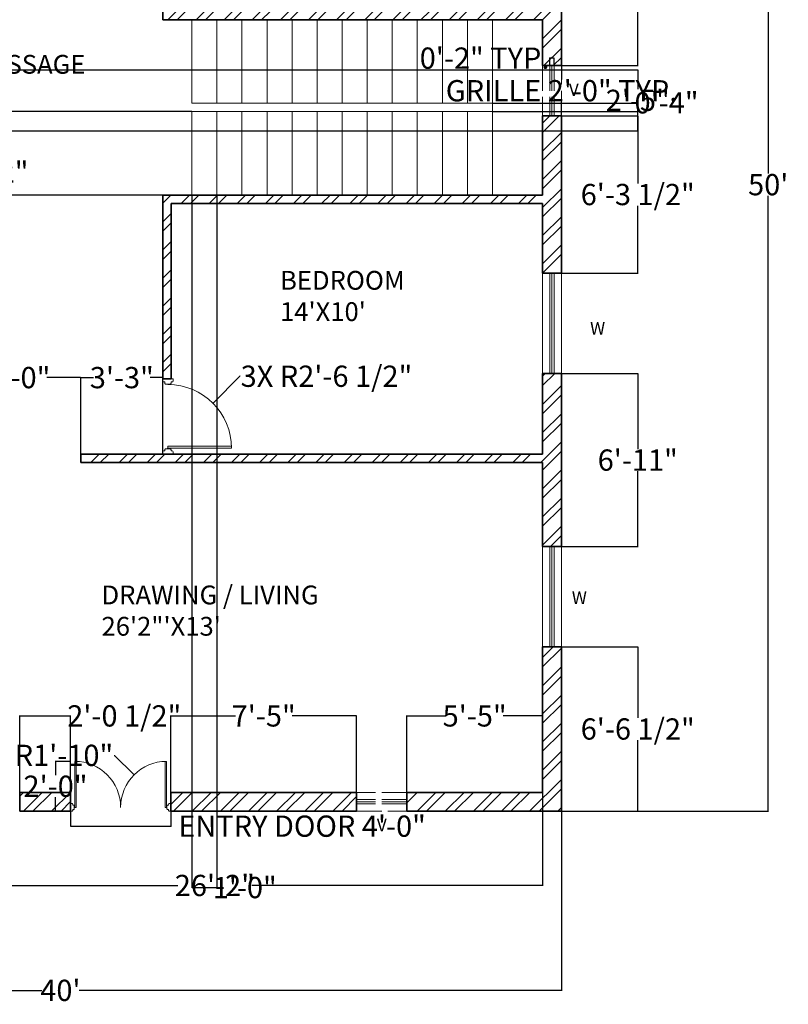
# Model space of a CAD drawing. Units: inches. Extents: x 1583 to 2239, y 1430 to 2174.
# Tile 4 of 5: x 1871 to 2239, y 1430 to 1902. Entities that reach past the tile are written whole.
import ezdxf

# ---------------------------------------------------------------- set-up
doc = ezdxf.new("R2010")
doc.units = ezdxf.units.IN
doc.linetypes.add('ACAD_ISO02W100', pattern=[15, 12, -3])
for name, color, linetype, lineweight in [('00 FURNITURE', 15, 'Continuous', 15), ('A-ANNO-DIMS', 2, 'Continuous', 18), ('A-ANNO-TEXT', 7, 'Continuous', 18), ('A-AREA-IDEN', 7, 'Continuous', 25), ('A-DOOR', 3, 'Continuous', 18), ('A-FLOR-STRS', 7, 'Continuous', 18), ('A-GLAZ-VENT', 6, 'ACAD_ISO02W100', 13), ('A-WALL-PATT', 252, 'Continuous', 13), ('WALL', 7, 'Continuous', 35), ('WINDOW', 160, 'Continuous', 18)]:
    doc.layers.add(name, color=color, linetype=linetype, lineweight=lineweight)
doc.styles.get("Standard").update_dxf_attribs({"font": 'arial.ttf'})
doc.dimstyles.get("Standard").update_dxf_attribs({"dimtxt": 10.18, "dimasz": 0.18, "dimexe": 0.18, "dimexo": 0.0625, "dimgap": 0.09, "dimtad": 0, "dimtih": 1, "dimtoh": 1, "dimdec": 0, "dimzin": 0, "dimdsep": 46, "dimlunit": 3, "dimtxsty": 'Standard', "dimcen": 0.09, "dimadec": 0, "dimazin": 0, "dimtfac": 1, "dimtdec": 0, "dimtofl": 0, "dimtmove": 0, "dimatfit": 3, "dimfxl": 1, "dimtolj": 1, "dimtzin": 0, "dimarcsym": 0})

# ---------------------------------------------------------------- blocks, each defined once
blk = doc.blocks.new('DDD')
at = {"layer": '00 FURNITURE'}
for p, q in [((-12579.77, -15859.53), (-12579.77, -15829.05)), ((-12578.77, -15859.53), (-12578.77, -15829.03)), ((-12612.02, -15857.03), (-12612.02, -15862.03)), ((-12611.02, -15857.03), (-12612.02, -15857.03)), ((-12610.52, -15858.03), (-12610.52, -15857.53)), ((-12610.52, -15861.53), (-12610.52, -15861.03)), ((-12578.77, -15859.53), (-12579.77, -15859.53)), ((-12577.52, -15858.03), (-12577.52, -15857.53)), ((-12577.52, -15861.53), (-12577.52, -15861.03)), ((-12577.02, -15857.03), (-12576.02, -15857.03)), ((-12576.02, -15857.03), (-12576.02, -15862.03)), ((-12612.02, -15862.03), (-12611.02, -15862.03)), ((-12576.02, -15862.03), (-12577.02, -15862.03))]:
    blk.add_line(p, q, dxfattribs=at)
for points in [[(-12610.52, -15861.03), (-12610.02, -15861.03, 0.414214), (-12609.52, -15860.53), (-12609.52, -15858.53, 0.414214), (-12610.02, -15858.03), (-12610.52, -15858.03)], [(-12577.52, -15861.03), (-12578.02, -15861.03, -0.414214), (-12578.52, -15860.53), (-12578.52, -15858.53, -0.414214), (-12578.02, -15858.03), (-12577.52, -15858.03)]]:
    blk.add_lwpolyline(points, format="xyb", dxfattribs=at)
for centre, radius, start, end in [((-12578.77, -15859.53), 30.5, 90, 180), ((-12611.02, -15857.53), 0.5, 0, 90), ((-12577.02, -15857.53), 0.5, 90, 180), ((-12611.02, -15861.53), 0.5, 270, 0), ((-12577.02, -15861.53), 0.5, 180, 270)]:
    blk.add_arc(centre, radius, start, end, dxfattribs=at)
blk = doc.blocks.new('*D3')
at = {"layer": 'A-ANNO-DIMS', "color": 0, "lineweight": -2, "transparency": 16777216}
for p, q in [((1807.53, 1531.58), (1807.53, 1486.86)), ((2121.53, 1531.58), (2121.53, 1486.86)), ((1807.71, 1487.04), (1946.87, 1487.04)), ((2121.35, 1487.04), (1982.19, 1487.04))]:
    blk.add_line(p, q, dxfattribs=at)
at = {"layer": 'A-ANNO-DIMS', "color": 0, "transparency": 16777216}
for points in [[(1807.71, 1487.07), (1807.71, 1487.01), (1807.53, 1487.04)], [(2121.35, 1487.07), (2121.35, 1487.01), (2121.53, 1487.04)]]:
    blk.add_solid(points, dxfattribs=at)
at = {"layer": 'Defpoints', "color": 0, "transparency": 16777216}
for p in [(1807.53, 1531.64), (2121.53, 1531.64), (2121.53, 1487.04)]:
    blk.add_point(p, dxfattribs=at)
at = {"layer": 'A-ANNO-DIMS', "color": 0, "transparency": 16777216, "insert": (1964.53, 1487.04), "char_height": 10.18, "attachment_point": 5}
blk.add_mtext('\\A1;26\'-2"', dxfattribs=at)
blk = doc.blocks.new('PUJA')
at = {"layer": '00 FURNITURE'}
for p, q in [((-1941.8, -16091.75), (-1938.89, -16091.75)), ((-1941.8, -16092.33), (-1941.8, -16091.75)), ((-1938.89, -16091.75), (-1938.89, -16092.33)), ((-1940.35, -16093.35), (-1958.14, -16093.35)), ((-1940.35, -16093.93), (-1958.13, -16093.93)), ((-1941.22, -16092.62), (-1941.51, -16092.62)), ((-1940.35, -16093.35), (-1940.35, -16093.93)), ((-1939.18, -16092.62), (-1939.47, -16092.62)), ((-1940.35, -16128.93), (-1958.14, -16128.93)), ((-1940.35, -16128.35), (-1958.13, -16128.35)), ((-1941.8, -16129.96), (-1941.8, -16130.54)), ((-1941.22, -16129.66), (-1941.51, -16129.66)), ((-1940.35, -16128.93), (-1940.35, -16128.35)), ((-1939.18, -16129.66), (-1939.47, -16129.66)), ((-1938.89, -16130.54), (-1938.89, -16129.96)), ((-1941.8, -16130.54), (-1938.89, -16130.54))]:
    blk.add_line(p, q, dxfattribs=at)
for points in [[(-1939.47, -16092.62), (-1939.47, -16092.91, -0.414214), (-1939.76, -16093.21), (-1940.93, -16093.21, -0.414214), (-1941.22, -16092.91), (-1941.22, -16092.62)], [(-1939.47, -16129.66), (-1939.47, -16129.37, 0.414214), (-1939.76, -16129.08), (-1940.93, -16129.08, 0.414214), (-1941.22, -16129.37), (-1941.22, -16129.66)]]:
    blk.add_lwpolyline(points, format="xyb", dxfattribs=at)
for centre, radius, start, end in [((-1940.35, -16093.35), 17.79, 180, 270), ((-1941.51, -16092.33), 0.292, 180, 270), ((-1939.18, -16092.33), 0.292, 270, 0), ((-1940.35, -16128.93), 17.79, 90, 180), ((-1941.51, -16129.96), 0.292, 90, 180), ((-1939.18, -16129.96), 0.292, 0, 90)]:
    blk.add_arc(centre, radius, start, end, dxfattribs=at)
blk = doc.blocks.new('*D9')
at = {"layer": 'A-ANNO-DIMS', "color": 0, "lineweight": -2, "transparency": 16777216}
for p, q in [((1650.53, 1522.58), (1650.53, 1436.63)), ((2130.53, 1522.58), (2130.53, 1436.63)), ((1650.71, 1436.81), (1881.6, 1436.81)), ((2130.35, 1436.81), (1899.47, 1436.81))]:
    blk.add_line(p, q, dxfattribs=at)
at = {"layer": 'A-ANNO-DIMS', "color": 0, "transparency": 16777216}
for points in [[(1650.71, 1436.84), (1650.71, 1436.78), (1650.53, 1436.81)], [(2130.35, 1436.84), (2130.35, 1436.78), (2130.53, 1436.81)]]:
    blk.add_solid(points, dxfattribs=at)
at = {"layer": 'Defpoints', "color": 0, "transparency": 16777216}
for p in [(1650.53, 1522.64), (2130.53, 1522.64), (2130.53, 1436.81)]:
    blk.add_point(p, dxfattribs=at)
at = {"layer": 'A-ANNO-DIMS', "color": 0, "transparency": 16777216, "insert": (1890.53, 1436.81), "char_height": 10.18, "attachment_point": 5}
blk.add_mtext("\\A1;40'", dxfattribs=at)
blk = doc.blocks.new('*D10')
at = {"layer": 'A-ANNO-DIMS', "color": 0, "lineweight": -2, "transparency": 16777216}
for p, q in [((2130.59, 2122.64), (2229.81, 2122.64)), ((2229.63, 2122.46), (2229.63, 1827.93)), ((2229.63, 1522.82), (2229.63, 1817.35)), ((2130.59, 1522.64), (2229.81, 1522.64))]:
    blk.add_line(p, q, dxfattribs=at)
at = {"layer": 'A-ANNO-DIMS', "color": 0, "transparency": 16777216}
for points in [[(2229.6, 2122.46), (2229.66, 2122.46), (2229.63, 2122.64)], [(2229.6, 1522.82), (2229.66, 1522.82), (2229.63, 1522.64)]]:
    blk.add_solid(points, dxfattribs=at)
at = {"layer": 'Defpoints', "color": 0, "transparency": 16777216}
for p in [(2130.53, 2122.64), (2130.53, 1522.64), (2229.63, 1522.64)]:
    blk.add_point(p, dxfattribs=at)
at = {"layer": 'A-ANNO-DIMS', "color": 0, "transparency": 16777216, "insert": (2229.63, 1822.64), "char_height": 10.18, "attachment_point": 5}
blk.add_mtext("\\A1;50'", dxfattribs=at)
blk = doc.blocks.new('WIN-SASH-48IN')
for p, q in [((48, 2), (0, 2)), ((48, 1), (0, 1)), ((48, 0), (0, 0))]:
    blk.add_line(p, q)
blk = doc.blocks.new('VENT-GRILLE-24IN')
for p, q in [((24, 2), (0, 2)), ((24, 1), (0, 1)), ((24, 0), (0, 0))]:
    blk.add_line(p, q)
blk = doc.blocks.new('*D15')
at = {"layer": 'A-ANNO-DIMS', "color": 0, "lineweight": -2, "transparency": 16777216}
for p, q in [((2127.09, 1879.63), (2130.81, 1879.63)), ((2130.63, 1879.45), (2130.63, 1872.98)), ((2130.63, 1855.81), (2130.63, 1862.27)), ((2127.09, 1855.63), (2130.81, 1855.63))]:
    blk.add_line(p, q, dxfattribs=at)
at = {"layer": 'A-ANNO-DIMS', "color": 0, "transparency": 16777216}
for points in [[(2130.6, 1879.45), (2130.66, 1879.45), (2130.63, 1879.63)], [(2130.6, 1855.81), (2130.66, 1855.81), (2130.63, 1855.63)]]:
    blk.add_solid(points, dxfattribs=at)
at = {"layer": 'Defpoints', "color": 0, "transparency": 16777216}
for p in [(2127.03, 1879.63), (2130.63, 1879.63), (2127.03, 1855.63)]:
    blk.add_point(p, dxfattribs=at)
at = {"layer": 'A-ANNO-DIMS', "color": 0, "transparency": 16777216, "insert": (2130.63, 1867.63), "char_height": 10.18, "attachment_point": 5}
blk.add_mtext('\\A1;GRILLE 2\'-0" TYP.', dxfattribs=at)
blk = doc.blocks.new('*D16')
at = {"layer": 'A-ANNO-DIMS', "color": 0, "lineweight": -2, "transparency": 16777216}
for p, q in [((2125.03, 1883.23), (2124.85, 1883.23)), ((2125.03, 1879.69), (2125.03, 1883.41)), ((2126.85, 1883.23), (2125.21, 1883.23)), ((2127.03, 1879.69), (2127.03, 1883.41))]:
    blk.add_line(p, q, dxfattribs=at)
at = {"layer": 'A-ANNO-DIMS', "color": 0, "transparency": 16777216}
for points in [[(2125.21, 1883.26), (2125.21, 1883.2), (2125.03, 1883.23)], [(2126.85, 1883.26), (2126.85, 1883.2), (2127.03, 1883.23)]]:
    blk.add_solid(points, dxfattribs=at)
at = {"layer": 'Defpoints', "color": 0, "transparency": 16777216}
for p in [(2125.03, 1883.23), (2125.03, 1879.63), (2127.03, 1879.63)]:
    blk.add_point(p, dxfattribs=at)
at = {"layer": 'A-ANNO-DIMS', "color": 0, "transparency": 16777216, "insert": (2093.74, 1883.23), "char_height": 10.18, "attachment_point": 5}
blk.add_mtext('\\A1;0\'-2" TYP.', dxfattribs=at)
blk = doc.blocks.new('*D27')
at = {"layer": 'A-ANNO-DIMS', "color": 0, "lineweight": -2, "transparency": 16777216}
for p, q in [((1895.39, 1522.58), (1895.39, 1515.26)), ((1943.39, 1522.58), (1943.39, 1515.26)), ((1895.57, 1515.44), (1943.21, 1515.44)), ((1943.39, 1515.44), (1943.57, 1515.44))]:
    blk.add_line(p, q, dxfattribs=at)
at = {"layer": 'A-ANNO-DIMS', "color": 0, "transparency": 16777216}
for points in [[(1895.57, 1515.47), (1895.57, 1515.41), (1895.39, 1515.44)], [(1943.21, 1515.47), (1943.21, 1515.41), (1943.39, 1515.44)]]:
    blk.add_solid(points, dxfattribs=at)
at = {"layer": 'Defpoints', "color": 0, "transparency": 16777216}
for p in [(1895.39, 1522.64), (1943.39, 1522.64), (1943.39, 1515.44)]:
    blk.add_point(p, dxfattribs=at)
at = {"layer": 'A-ANNO-DIMS', "color": 0, "transparency": 16777216, "insert": (2006.31, 1515.44), "char_height": 10.18, "attachment_point": 5}
blk.add_mtext('\\A1;ENTRY DOOR 4\'-0"', dxfattribs=at)
blk = doc.blocks.new('*D28')
at = {"layer": 'A-ANNO-DIMS', "color": 0, "lineweight": -2, "transparency": 16777216}
for p, q in [((1895.33, 1546.46), (1888.01, 1546.46)), ((1888.19, 1546.28), (1888.19, 1539.84)), ((1888.19, 1522.82), (1888.19, 1529.26)), ((1895.33, 1522.64), (1888.01, 1522.64))]:
    blk.add_line(p, q, dxfattribs=at)
at = {"layer": 'A-ANNO-DIMS', "color": 0, "transparency": 16777216}
for points in [[(1888.16, 1546.28), (1888.22, 1546.28), (1888.19, 1546.46)], [(1888.16, 1522.82), (1888.22, 1522.82), (1888.19, 1522.64)]]:
    blk.add_solid(points, dxfattribs=at)
at = {"layer": 'Defpoints', "color": 0, "transparency": 16777216}
for p in [(1895.39, 1546.46), (1888.19, 1522.64), (1895.39, 1522.64)]:
    blk.add_point(p, dxfattribs=at)
at = {"layer": 'A-ANNO-DIMS', "color": 0, "transparency": 16777216, "insert": (1888.19, 1534.55), "char_height": 10.18, "attachment_point": 5}
blk.add_mtext('\\A1;2\'-0"', dxfattribs=at)
blk = doc.blocks.new('*D33')
at = {"layer": 'A-ANNO-DIMS', "color": 0, "lineweight": -2, "transparency": 16777216}
for p, q in [((2056.46, 1531.7), (2056.46, 1568.42)), ((2056.64, 1568.24), (2075.38, 1568.24)), ((2121.35, 1568.24), (2102.62, 1568.24)), ((2121.53, 1531.7), (2121.53, 1568.42))]:
    blk.add_line(p, q, dxfattribs=at)
at = {"layer": 'A-ANNO-DIMS', "color": 0, "transparency": 16777216}
for points in [[(2056.64, 1568.27), (2056.64, 1568.21), (2056.46, 1568.24)], [(2121.35, 1568.27), (2121.35, 1568.21), (2121.53, 1568.24)]]:
    blk.add_solid(points, dxfattribs=at)
at = {"layer": 'Defpoints', "color": 0, "transparency": 16777216}
for p in [(2121.53, 1568.24), (2056.46, 1531.64), (2121.53, 1531.64)]:
    blk.add_point(p, dxfattribs=at)
at = {"layer": 'A-ANNO-DIMS', "color": 0, "transparency": 16777216, "insert": (2089, 1568.24), "char_height": 10.18, "attachment_point": 5}
blk.add_mtext('\\A1;5\'-5"', dxfattribs=at)
blk = doc.blocks.new('*D34')
at = {"layer": 'A-ANNO-DIMS', "color": 0, "lineweight": -2, "transparency": 16777216}
for p, q in [((1871.02, 1531.7), (1871.02, 1568.42)), ((1871.2, 1568.24), (1895.21, 1568.24)), ((1895.39, 1531.7), (1895.39, 1568.42)), ((1895.39, 1568.24), (1895.57, 1568.24))]:
    blk.add_line(p, q, dxfattribs=at)
at = {"layer": 'A-ANNO-DIMS', "color": 0, "transparency": 16777216}
for points in [[(1871.2, 1568.27), (1871.2, 1568.21), (1871.02, 1568.24)], [(1895.21, 1568.27), (1895.21, 1568.21), (1895.39, 1568.24)]]:
    blk.add_solid(points, dxfattribs=at)
at = {"layer": 'Defpoints', "color": 0, "transparency": 16777216}
for p in [(1895.39, 1568.24), (1871.02, 1531.64), (1895.39, 1531.64)]:
    blk.add_point(p, dxfattribs=at)
at = {"layer": 'A-ANNO-DIMS', "color": 0, "transparency": 16777216, "insert": (1921.14, 1568.24), "char_height": 10.18, "attachment_point": 5}
blk.add_mtext('\\A1;2\'-0 1/2"', dxfattribs=at)
blk = doc.blocks.new('*D35')
at = {"layer": 'A-ANNO-DIMS', "color": 0, "lineweight": -2, "transparency": 16777216}
for p, q in [((1943.39, 1531.7), (1943.39, 1568.42)), ((1943.57, 1568.24), (1974.35, 1568.24)), ((2032.28, 1568.24), (2001.51, 1568.24)), ((2032.46, 1531.7), (2032.46, 1568.42))]:
    blk.add_line(p, q, dxfattribs=at)
at = {"layer": 'A-ANNO-DIMS', "color": 0, "transparency": 16777216}
for points in [[(1943.57, 1568.27), (1943.57, 1568.21), (1943.39, 1568.24)], [(2032.28, 1568.27), (2032.28, 1568.21), (2032.46, 1568.24)]]:
    blk.add_solid(points, dxfattribs=at)
at = {"layer": 'Defpoints', "color": 0, "transparency": 16777216}
for p in [(2032.46, 1568.24), (1943.39, 1531.64), (2032.46, 1531.64)]:
    blk.add_point(p, dxfattribs=at)
at = {"layer": 'A-ANNO-DIMS', "color": 0, "transparency": 16777216, "insert": (1987.93, 1568.24), "char_height": 10.18, "attachment_point": 5}
blk.add_mtext('\\A1;7\'-5"', dxfattribs=at)
blk = doc.blocks.new('*D40')
at = {"layer": 'A-ANNO-DIMS', "color": 0, "lineweight": -2, "transparency": 16777216}
for p, q in [((2130.59, 1601.31), (2167.31, 1601.31)), ((2167.13, 1601.13), (2167.13, 1567.33)), ((2167.13, 1522.82), (2167.13, 1556.62)), ((2130.59, 1522.64), (2167.31, 1522.64))]:
    blk.add_line(p, q, dxfattribs=at)
at = {"layer": 'A-ANNO-DIMS', "color": 0, "transparency": 16777216}
for points in [[(2167.1, 1601.13), (2167.16, 1601.13), (2167.13, 1601.31)], [(2167.1, 1522.82), (2167.16, 1522.82), (2167.13, 1522.64)]]:
    blk.add_solid(points, dxfattribs=at)
at = {"layer": 'Defpoints', "color": 0, "transparency": 16777216}
for p in [(2130.53, 1601.31), (2167.13, 1601.31), (2130.53, 1522.64)]:
    blk.add_point(p, dxfattribs=at)
at = {"layer": 'A-ANNO-DIMS', "color": 0, "transparency": 16777216, "insert": (2167.13, 1561.97), "char_height": 10.18, "attachment_point": 5}
blk.add_mtext('\\A1;6\'-6 1/2"', dxfattribs=at)
blk = doc.blocks.new('*D41')
at = {"layer": 'A-ANNO-DIMS', "color": 0, "lineweight": -2, "transparency": 16777216}
for p, q in [((2130.59, 1732.2), (2167.31, 1732.2)), ((2167.13, 1732.02), (2167.13, 1696.04)), ((2167.13, 1649.49), (2167.13, 1685.47)), ((2130.59, 1649.31), (2167.31, 1649.31))]:
    blk.add_line(p, q, dxfattribs=at)
at = {"layer": 'A-ANNO-DIMS', "color": 0, "transparency": 16777216}
for points in [[(2167.1, 1732.02), (2167.16, 1732.02), (2167.13, 1732.2)], [(2167.1, 1649.49), (2167.16, 1649.49), (2167.13, 1649.31)]]:
    blk.add_solid(points, dxfattribs=at)
at = {"layer": 'Defpoints', "color": 0, "transparency": 16777216}
for p in [(2130.53, 1732.2), (2167.13, 1732.2), (2130.53, 1649.31)]:
    blk.add_point(p, dxfattribs=at)
at = {"layer": 'A-ANNO-DIMS', "color": 0, "transparency": 16777216, "insert": (2167.13, 1690.75), "char_height": 10.18, "attachment_point": 5}
blk.add_mtext('\\A1;6\'-11"', dxfattribs=at)
blk = doc.blocks.new('*D42')
at = {"layer": 'A-ANNO-DIMS', "color": 0, "lineweight": -2, "transparency": 16777216}
for p, q in [((2130.59, 1855.63), (2167.31, 1855.63)), ((2167.13, 1855.45), (2167.13, 1823.27)), ((2167.13, 1780.38), (2167.13, 1812.55)), ((2130.59, 1780.2), (2167.31, 1780.2))]:
    blk.add_line(p, q, dxfattribs=at)
at = {"layer": 'A-ANNO-DIMS', "color": 0, "transparency": 16777216}
for points in [[(2167.1, 1855.45), (2167.16, 1855.45), (2167.13, 1855.63)], [(2167.1, 1780.38), (2167.16, 1780.38), (2167.13, 1780.2)]]:
    blk.add_solid(points, dxfattribs=at)
at = {"layer": 'Defpoints', "color": 0, "transparency": 16777216}
for p in [(2130.53, 1855.63), (2167.13, 1855.63), (2130.53, 1780.2)]:
    blk.add_point(p, dxfattribs=at)
at = {"layer": 'A-ANNO-DIMS', "color": 0, "transparency": 16777216, "insert": (2167.13, 1817.91), "char_height": 10.18, "attachment_point": 5}
blk.add_mtext('\\A1;6\'-3 1/2"', dxfattribs=at)
blk = doc.blocks.new('*D43')
at = {"layer": 'A-ANNO-DIMS', "color": 0, "lineweight": -2, "transparency": 16777216}
for p, q in [((2130.59, 1965.82), (2167.31, 1965.82)), ((2167.13, 1965.64), (2167.13, 1927.92)), ((2167.13, 1879.81), (2167.13, 1917.52)), ((2130.59, 1879.63), (2167.31, 1879.63))]:
    blk.add_line(p, q, dxfattribs=at)
at = {"layer": 'A-ANNO-DIMS', "color": 0, "transparency": 16777216}
for points in [[(2167.1, 1965.64), (2167.16, 1965.64), (2167.13, 1965.82)], [(2167.1, 1879.81), (2167.16, 1879.81), (2167.13, 1879.63)]]:
    blk.add_solid(points, dxfattribs=at)
at = {"layer": 'Defpoints', "color": 0, "transparency": 16777216}
for p in [(2130.53, 1965.82), (2167.13, 1965.82), (2130.53, 1879.63)]:
    blk.add_point(p, dxfattribs=at)
at = {"layer": 'A-ANNO-DIMS', "color": 0, "transparency": 16777216, "insert": (2167.13, 1922.72), "char_height": 10.18, "attachment_point": 5}
blk.add_mtext('\\A1;7\'-2"', dxfattribs=at)
blk = doc.blocks.new('*D44')
at = {"layer": 'A-ANNO-DIMS', "color": 0, "lineweight": -2, "transparency": 16777216}
for p, q in [((1953.47, 1857.64), (1613.75, 1857.64)), ((1613.93, 1857.46), (1613.93, 1842.93)), ((1613.93, 1817.82), (1613.93, 1832.35)), ((1953.47, 1817.64), (1613.75, 1817.64))]:
    blk.add_line(p, q, dxfattribs=at)
at = {"layer": 'A-ANNO-DIMS', "color": 0, "transparency": 16777216}
for points in [[(1613.9, 1857.46), (1613.96, 1857.46), (1613.93, 1857.64)], [(1613.9, 1817.82), (1613.96, 1817.82), (1613.93, 1817.64)]]:
    blk.add_solid(points, dxfattribs=at)
at = {"layer": 'Defpoints', "color": 0, "transparency": 16777216}
for p in [(1613.93, 1857.64), (1953.53, 1857.64), (1953.53, 1817.64)]:
    blk.add_point(p, dxfattribs=at)
at = {"layer": 'A-ANNO-DIMS', "color": 0, "transparency": 16777216, "insert": (1613.93, 1837.64), "char_height": 10.18, "attachment_point": 5}
blk.add_mtext('\\A1;3\'-4"', dxfattribs=at)
blk = doc.blocks.new('*D45')
at = {"layer": 'A-ANNO-DIMS', "color": 0, "lineweight": -2, "transparency": 16777216}
for p, q in [((2097.59, 1861.64), (2167.31, 1861.64)), ((2167.13, 1861.64), (2167.13, 1861.82)), ((2167.13, 1861.82), (2167.31, 1861.82)), ((2167.13, 1857.82), (2167.13, 1861.46)), ((2097.59, 1857.64), (2167.31, 1857.64))]:
    blk.add_line(p, q, dxfattribs=at)
at = {"layer": 'A-ANNO-DIMS', "color": 0, "transparency": 16777216}
for points in [[(2167.1, 1861.46), (2167.16, 1861.46), (2167.13, 1861.64)], [(2167.1, 1857.82), (2167.16, 1857.82), (2167.13, 1857.64)]]:
    blk.add_solid(points, dxfattribs=at)
at = {"layer": 'Defpoints', "color": 0, "transparency": 16777216}
for p in [(2097.53, 1861.64), (2167.13, 1861.64), (2097.53, 1857.64)]:
    blk.add_point(p, dxfattribs=at)
at = {"layer": 'A-ANNO-DIMS', "color": 0, "transparency": 16777216, "insert": (2180.93, 1861.82), "char_height": 10.18, "attachment_point": 5}
blk.add_mtext('\\A1;0\'-4"', dxfattribs=at)
blk = doc.blocks.new('*D47')
at = {"layer": 'A-ANNO-DIMS', "color": 0, "lineweight": -2, "transparency": 16777216}
for p, q in [((1953.53, 1817.58), (1953.53, 1485.86)), ((1965.53, 1817.58), (1965.53, 1485.86)), ((1953.71, 1486.04), (1965.35, 1486.04)), ((1965.53, 1486.04), (1965.71, 1486.04))]:
    blk.add_line(p, q, dxfattribs=at)
at = {"layer": 'A-ANNO-DIMS', "color": 0, "transparency": 16777216}
for points in [[(1953.71, 1486.07), (1953.71, 1486.01), (1953.53, 1486.04)], [(1965.35, 1486.07), (1965.35, 1486.01), (1965.53, 1486.04)]]:
    blk.add_solid(points, dxfattribs=at)
at = {"layer": 'Defpoints', "color": 0, "transparency": 16777216}
for p in [(1953.53, 1817.64), (1965.53, 1817.64), (1965.53, 1486.04)]:
    blk.add_point(p, dxfattribs=at)
at = {"layer": 'A-ANNO-DIMS', "color": 0, "transparency": 16777216, "insert": (1978.85, 1486.04), "char_height": 10.18, "attachment_point": 5}
blk.add_mtext('\\A1;1\'-0"', dxfattribs=at)
blk = doc.blocks.new('*D51')
at = {"layer": 'A-ANNO-DIMS', "color": 0, "lineweight": -2, "transparency": 16777216}
for p, q in [((1840.39, 1693.7), (1840.39, 1730.42)), ((1840.57, 1730.24), (1856.77, 1730.24)), ((1900.21, 1730.24), (1884.01, 1730.24)), ((1900.39, 1693.7), (1900.39, 1730.42))]:
    blk.add_line(p, q, dxfattribs=at)
at = {"layer": 'A-ANNO-DIMS', "color": 0, "transparency": 16777216}
for points in [[(1840.57, 1730.27), (1840.57, 1730.21), (1840.39, 1730.24)], [(1900.21, 1730.27), (1900.21, 1730.21), (1900.39, 1730.24)]]:
    blk.add_solid(points, dxfattribs=at)
at = {"layer": 'Defpoints', "color": 0, "transparency": 16777216}
for p in [(1900.39, 1730.24), (1840.39, 1693.64), (1900.39, 1693.64)]:
    blk.add_point(p, dxfattribs=at)
at = {"layer": 'A-ANNO-DIMS', "color": 0, "transparency": 16777216, "insert": (1870.39, 1730.24), "char_height": 10.18, "attachment_point": 5}
blk.add_mtext('\\A1;5\'-0"', dxfattribs=at)
blk = doc.blocks.new('*D56')
at = {"layer": 'A-ANNO-DIMS', "color": 0, "lineweight": -2, "transparency": 16777216}
for p, q in [((1803.59, 1877.64), (2167.31, 1877.64)), ((2167.13, 1877.46), (2167.13, 1868.3)), ((2167.13, 1848.57), (2167.13, 1857.73)), ((1802.65, 1848.39), (2167.31, 1848.39))]:
    blk.add_line(p, q, dxfattribs=at)
at = {"layer": 'A-ANNO-DIMS', "color": 0, "transparency": 16777216}
for points in [[(2167.1, 1877.46), (2167.16, 1877.46), (2167.13, 1877.64)], [(2167.1, 1848.57), (2167.16, 1848.57), (2167.13, 1848.39)]]:
    blk.add_solid(points, dxfattribs=at)
at = {"layer": 'Defpoints', "color": 0, "transparency": 16777216}
for p in [(1803.53, 1877.64), (1802.59, 1848.39), (2167.13, 1848.39)]:
    blk.add_point(p, dxfattribs=at)
at = {"layer": 'A-ANNO-DIMS', "color": 0, "transparency": 16777216, "insert": (2167.13, 1863.01), "char_height": 10.18, "attachment_point": 5}
blk.add_mtext('\\A1;2\'-5"', dxfattribs=at)
blk = doc.blocks.new('*D57')
at = {"layer": 'A-ANNO-DIMS', "color": 0, "lineweight": -2, "transparency": 16777216}
for p, q in [((1900.39, 1693.7), (1900.39, 1730.42)), ((1900.57, 1730.24), (1906.34, 1730.24)), ((1939.35, 1730.24), (1933.58, 1730.24)), ((1939.53, 1693.7), (1939.53, 1730.42))]:
    blk.add_line(p, q, dxfattribs=at)
at = {"layer": 'A-ANNO-DIMS', "color": 0, "transparency": 16777216}
for points in [[(1900.57, 1730.27), (1900.57, 1730.21), (1900.39, 1730.24)], [(1939.35, 1730.27), (1939.35, 1730.21), (1939.53, 1730.24)]]:
    blk.add_solid(points, dxfattribs=at)
at = {"layer": 'Defpoints', "color": 0, "transparency": 16777216}
for p in [(1939.53, 1730.24), (1900.39, 1693.64), (1939.53, 1693.64)]:
    blk.add_point(p, dxfattribs=at)
at = {"layer": 'A-ANNO-DIMS', "color": 0, "transparency": 16777216, "insert": (1919.96, 1730.24), "char_height": 10.18, "attachment_point": 5}
blk.add_mtext('\\A1;3\'-3"', dxfattribs=at)
blk = doc.blocks.new('*D61')
at = {"layer": 'A-ANNO-DIMS', "color": 0, "lineweight": -2, "transparency": 16777216}
for p, q in [((1976.54, 1730.9), (1963.73, 1718.08)), ((1976.72, 1730.9), (1976.54, 1730.9)), ((1941.94, 1696.39), (1942.12, 1696.39)), ((1942.03, 1696.3), (1942.03, 1696.48))]:
    blk.add_line(p, q, dxfattribs=at)
at = {"layer": 'A-ANNO-DIMS', "color": 0, "transparency": 16777216}
blk.add_solid([(1963.7, 1718.1), (1963.75, 1718.06), (1963.6, 1717.96)], dxfattribs=at)
at = {"layer": 'Defpoints', "color": 0, "transparency": 16777216}
for p in [(1963.6, 1717.96), (1942.03, 1696.39)]:
    blk.add_point(p, dxfattribs=at)
at = {"layer": 'A-ANNO-DIMS', "color": 0, "transparency": 16777216, "insert": (2018, 1730.9), "char_height": 10.18, "attachment_point": 5}
blk.add_mtext('\\A1;3X R2\'-6 1/2"', dxfattribs=at)
blk = doc.blocks.new('*D63')
at = {"layer": 'A-ANNO-DIMS', "color": 0, "lineweight": -2, "transparency": 16777216}
for p, q in [((1916.32, 1549.35), (1916.5, 1549.35)), ((1916.5, 1549.35), (1925.71, 1540.14)), ((1941.32, 1524.44), (1941.5, 1524.44)), ((1941.41, 1524.35), (1941.41, 1524.53))]:
    blk.add_line(p, q, dxfattribs=at)
at = {"layer": 'A-ANNO-DIMS', "color": 0, "transparency": 16777216}
blk.add_solid([(1925.73, 1540.16), (1925.69, 1540.12), (1925.84, 1540.01)], dxfattribs=at)
at = {"layer": 'Defpoints', "color": 0, "transparency": 16777216}
for p in [(1925.84, 1540.01), (1941.41, 1524.44)]:
    blk.add_point(p, dxfattribs=at)
at = {"layer": 'A-ANNO-DIMS', "color": 0, "transparency": 16777216, "insert": (1882.85, 1549.35), "char_height": 10.18, "attachment_point": 5}
blk.add_mtext('\\A1;2X R1\'-10"', dxfattribs=at)
blk = doc.blocks.new('*D65')
at = {"layer": 'A-ANNO-DIMS', "color": 0, "lineweight": -2, "transparency": 16777216}
for p, q in [((1784.89, 1841.88), (1785.07, 1841.88)), ((1784.98, 1841.79), (1784.98, 1841.97)), ((1792.63, 1828.66), (1789.85, 1833.46)), ((1792.81, 1828.66), (1792.63, 1828.66))]:
    blk.add_line(p, q, dxfattribs=at)
at = {"layer": 'A-ANNO-DIMS', "color": 0, "transparency": 16777216}
blk.add_solid([(1789.88, 1833.48), (1789.83, 1833.45), (1789.76, 1833.62)], dxfattribs=at)
at = {"layer": 'Defpoints', "color": 0, "transparency": 16777216}
for p in [(1784.98, 1841.88), (1789.76, 1833.62)]:
    blk.add_point(p, dxfattribs=at)
at = {"layer": 'A-ANNO-DIMS', "color": 0, "transparency": 16777216, "insert": (1834.11, 1828.66), "char_height": 10.18, "attachment_point": 5}
blk.add_mtext('\\A1;8X R0\'-9 1/2"', dxfattribs=at)

msp = doc.modelspace()

# ---------------------------------------------------------------- hatches: boundary and pattern name
at = {"layer": 'A-WALL-PATT'}
h = msp.add_hatch(dxfattribs=at)
h.set_pattern_fill('ANSI32', color=256)
h.paths.add_polyline_path([(1715.9, 2122.64), (1650.53, 2122.64), (1650.53, 1975.26), (1659.53, 1975.26), (1659.53, 1975.26), (1659.53, 2013.64), (1803.53, 2013.64), (1803.53, 1917.64), (1807.53, 1917.64), (1807.53, 2013.64), (1839.53, 2013.64), (1839.53, 2017.64), (1659.53, 2017.64), (1659.53, 2113.64), (1715.9, 2113.64)])
h.paths.add_polyline_path([(1893.86, 2122.64), (1763.9, 2122.64), (1763.9, 2113.64), (1875.53, 2113.64), (1875.53, 2013.64), (1879.53, 2013.64), (1879.53, 2037.64), (1909.53, 2037.64), (1909.53, 2041.64), (1879.53, 2041.64), (1879.53, 2113.64), (1893.86, 2113.64)])
h.paths.add_polyline_path([(1999.8, 2122.64), (1917.86, 2122.64), (1917.86, 2113.64), (1939.53, 2113.64), (1939.53, 2037.64), (1939.53, 1941.64), (1943.53, 1941.64), (1943.53, 2049.64), (2091.53, 2049.64), (2091.53, 2053.64), (1943.53, 2053.64), (1943.53, 2113.64), (1999.8, 2113.64)])
h.paths.add_polyline_path([(2130.53, 2122.64), (2023.8, 2122.64), (2023.8, 2113.64), (2121.53, 2113.64), (2121.53, 2049.64), (2121.53, 2013.82), (2130.53, 2013.82), (2130.53, 2013.82)])
h.paths.add_polyline_path([(2130.53, 1965.82), (2121.53, 1965.82), (2121.53, 1905.64), (1944.53, 1905.64), (1944.53, 1905.64), (1939.53, 1905.64), (1939.53, 1901.64), (2121.53, 1901.64), (2121.53, 1879.63), (2130.53, 1879.63)])
h.paths.add_polyline_path([(2130.53, 1855.63), (2121.53, 1855.63), (2121.53, 1817.64), (1939.53, 1817.64), (1939.53, 1729.64), (1943.53, 1729.64), (1943.53, 1813.64), (2121.53, 1813.64), (2121.53, 1780.2), (2130.53, 1780.2), (2130.53, 1780.2)])
h.paths.add_polyline_path([(2130.53, 1732.2), (2121.53, 1732.2), (2121.53, 1693.64), (1944.53, 1693.64), (1944.53, 1693.64), (1939.53, 1693.64), (1900.39, 1693.64), (1900.39, 1689.64), (2121.53, 1689.64), (2121.53, 1649.31), (2130.53, 1649.31), (2130.53, 1649.31)])
h.paths.add_polyline_path([(2130.53, 1601.31), (2121.53, 1601.31), (2121.53, 1531.64), (2056.46, 1531.64), (2056.46, 1522.64), (2130.53, 1522.64)])
h.paths.add_polyline_path([(2032.46, 1531.64), (1943.39, 1531.64), (1943.39, 1526.25), (1943.39, 1526.25), (1943.39, 1522.64), (2032.46, 1522.64)])
h.paths.add_polyline_path([(1895.39, 1531.64), (1871.02, 1531.64), (1871.02, 1522.64), (1895.39, 1522.64)])
h.paths.add_polyline_path([(1847.02, 1531.64), (1807.53, 1531.64), (1807.53, 1653.64), (1803.53, 1653.64), (1803.53, 1531.64), (1750.06, 1531.64), (1750.06, 1522.64), (1847.02, 1522.64)])
h.paths.add_polyline_path([(1702.06, 1531.64), (1659.53, 1531.64), (1659.53, 1587.56), (1650.53, 1587.56), (1650.53, 1522.64), (1702.06, 1522.64)])
h.paths.add_polyline_path([(1659.53, 1927.26), (1650.53, 1927.26), (1650.53, 1843.95), (1659.53, 1843.95), (1659.53, 1877.64)])
h.paths.add_polyline_path([(1659.53, 1801.64), (1807.53, 1801.64), (1807.53, 1881.64), (1689.53, 1881.64), (1689.53, 1877.64), (1803.53, 1877.64), (1803.53, 1805.64), (1659.53, 1805.64), (1659.53, 1819.95), (1650.53, 1819.95), (1650.53, 1766.08), (1659.53, 1766.08)])
h.paths.add_polyline_path([(1659.53, 1742.08), (1650.53, 1742.08), (1650.53, 1635.56), (1659.53, 1635.56), (1659.53, 1635.56), (1659.53, 1689.64), (1807.53, 1689.64), (1840.39, 1689.64), (1840.39, 1693.64), (1807.53, 1693.64), (1807.53, 1771.64), (1803.53, 1771.64), (1803.53, 1693.64), (1786.54, 1693.64), (1786.54, 1693.64), (1768.55, 1693.64), (1659.53, 1693.64), (1659.53, 1701.64)])

# ---------------------------------------------------------------- linework, layer by layer
at = {"layer": 'A-FLOR-STRS'}
for p, q in [((1953.53, 1901.64), (1953.53, 1861.64)), ((1965.53, 1901.64), (1965.53, 1861.64)), ((1977.53, 1901.64), (1977.53, 1861.64)), ((1989.53, 1901.64), (1989.53, 1861.64)), ((2001.53, 1901.64), (2001.53, 1861.64)), ((2013.53, 1901.64), (2013.53, 1861.64)), ((2025.53, 1901.64), (2025.53, 1861.64)), ((2037.53, 1901.64), (2037.53, 1861.64)), ((2049.53, 1901.64), (2049.53, 1861.64)), ((2061.53, 1901.64), (2061.53, 1861.64)), ((2073.53, 1901.64), (2073.53, 1861.64)), ((2085.53, 1901.64), (2085.53, 1861.64)), ((2097.53, 1901.64), (2097.53, 1817.64)), ((2097.53, 1861.64), (1953.53, 1861.64)), ((2097.53, 1857.64), (1953.53, 1857.64)), ((1953.53, 1857.64), (1953.53, 1817.64)), ((1965.53, 1857.64), (1965.53, 1817.64)), ((1977.53, 1857.64), (1977.53, 1817.64)), ((1989.53, 1857.64), (1989.53, 1817.64)), ((2001.53, 1857.64), (2001.53, 1817.64)), ((2013.53, 1857.64), (2013.53, 1817.64)), ((2025.53, 1857.64), (2025.53, 1817.64)), ((2037.53, 1857.64), (2037.53, 1817.64)), ((2049.53, 1857.64), (2049.53, 1817.64)), ((2061.53, 1857.64), (2061.53, 1817.64)), ((2073.53, 1857.64), (2073.53, 1817.64)), ((2085.53, 1857.64), (2085.53, 1817.64))]:
    msp.add_line(p, q, dxfattribs=at)
at = {"layer": 'A-GLAZ-VENT'}
for points in [[(2121.53, 1855.63), (2130.53, 1855.63), (2130.53, 1879.63), (2121.53, 1879.63)], [(2032.46, 1531.64), (2032.46, 1522.64), (2056.46, 1522.64), (2056.46, 1531.64)]]:
    msp.add_lwpolyline(points, close=True, dxfattribs=at)
at = {"layer": 'WALL'}
for p, q in [((2130.53, 1965.82), (2130.53, 1879.63)), ((1939.53, 1901.64), (1939.53, 1905.64)), ((1939.53, 1901.64), (2121.53, 1901.64)), ((2121.53, 1901.64), (2121.53, 1879.63)), ((2121.53, 1879.63), (2130.53, 1879.63)), ((2121.53, 1855.63), (2130.53, 1855.63)), ((2121.53, 1855.63), (2121.53, 1817.64)), ((2130.53, 1855.63), (2130.53, 1780.2)), ((1939.53, 1729.64), (1939.53, 1817.64)), ((1939.53, 1817.64), (2121.53, 1817.64)), ((1943.53, 1813.64), (2121.53, 1813.64)), ((1943.53, 1729.64), (1943.53, 1813.64)), ((2121.53, 1813.64), (2121.53, 1780.2)), ((2121.53, 1780.2), (2130.53, 1780.2)), ((2121.53, 1732.2), (2130.53, 1732.2)), ((2121.53, 1732.2), (2121.53, 1693.64)), ((2130.53, 1732.2), (2130.53, 1649.31)), ((1939.53, 1729.64), (1943.53, 1729.64)), ((1900.39, 1689.64), (1900.39, 1693.64)), ((1900.39, 1693.64), (1939.53, 1693.64)), ((1939.53, 1693.64), (2121.53, 1693.64)), ((1900.39, 1689.64), (2121.53, 1689.64)), ((2121.53, 1689.64), (2121.53, 1649.31)), ((2121.53, 1649.31), (2130.53, 1649.31)), ((2121.53, 1601.31), (2130.53, 1601.31)), ((2121.53, 1601.31), (2121.53, 1531.64)), ((2130.53, 1601.31), (2130.53, 1522.64)), ((1895.39, 1531.64), (1871.02, 1531.64)), ((1871.02, 1522.64), (1871.02, 1531.64)), ((1895.39, 1531.64), (1879.53, 1531.64)), ((1895.39, 1531.64), (1895.39, 1522.64)), ((1943.39, 1531.64), (1943.39, 1522.64)), ((2032.46, 1531.64), (1943.39, 1531.64)), ((2032.46, 1531.64), (1943.53, 1531.64)), ((2032.46, 1531.64), (2032.46, 1522.64)), ((2121.53, 1531.64), (2056.46, 1531.64)), ((2121.53, 1531.64), (2056.46, 1531.64)), ((2056.46, 1531.64), (2056.46, 1522.64)), ((1895.39, 1522.64), (1871.02, 1522.64)), ((2032.46, 1522.64), (1943.39, 1522.64)), ((2130.53, 1522.64), (2056.46, 1522.64))]:
    msp.add_line(p, q, dxfattribs=at)
at = {"layer": 'WINDOW'}
for p, q in [((2121.53, 1780.2), (2121.53, 1732.2)), ((2130.53, 1732.2), (2130.53, 1780.2)), ((2121.53, 1649.31), (2121.53, 1601.31)), ((2130.53, 1601.31), (2130.53, 1649.31))]:
    msp.add_line(p, q, dxfattribs=at)

# ---------------------------------------------------------------- block references
at = {"layer": 'A-DOOR', "rotation": 270}
msp.add_blockref('DDD', (17801.56, -10882.38), dxfattribs=at)
at = {"layer": 'A-DOOR', "xscale": 1.237379162154587, "yscale": 1.237379162154587, "zscale": 1.237379162154587, "rotation": 270.0000000034012}
msp.add_blockref('PUJA', (21854.98, -876.5), dxfattribs=at)
at = {"layer": 'A-GLAZ-VENT', "rotation": 89.99999999999883}
msp.add_blockref('VENT-GRILLE-24IN', (2127.03, 1855.63), dxfattribs=at)
at = {"layer": 'A-GLAZ-VENT'}
msp.add_blockref('VENT-GRILLE-24IN', (2032.46, 1526.14), dxfattribs=at)
at = {"layer": 'WINDOW', "rotation": 270.0000000000001}
for p in [(2125.03, 1780.2), (2125.03, 1649.31)]:
    msp.add_blockref('WIN-SASH-48IN', p, dxfattribs=at)

# ---------------------------------------------------------------- texts
at = {"layer": 'A-ANNO-TEXT', "char_height": 6, "attachment_point": 1}
for s, insert in [('V', (2134.15, 1871.08)), ('W', (2144.31, 1756.82)), ('W', (2135.56, 1627.84)), ('V', (2042.15, 1518.97))]:
    msp.add_mtext_dynamic_manual_height_columns(s, width=236.3031, gutter_width=12.5, heights=[0], dxfattribs=dict(at, insert=insert))
at = {"layer": 'A-AREA-IDEN', "char_height": 9, "attachment_point": 1}
for s, insert in [('PASSAGE ', (1849.48, 1884.77)), ("BEDROOM\\P14'X10'", (1995.76, 1781.33)), ('DRAWING / LIVING \\P26\'2"\'X13\'', (1910.24, 1630.66))]:
    msp.add_mtext_dynamic_manual_height_columns(s, width=172.7707, gutter_width=12.5, heights=[0], dxfattribs=dict(at, insert=insert))

# ---------------------------------------------------------------- dimensions: what is measured, and where the dimension line sits
at = {"layer": 'A-ANNO-DIMS'}
for base, p1, p2, angle, override, picture, middle in [((2229.63, 1522.64), (2130.53, 2122.64), (2130.53, 1522.64), 90, {"dimclrd": 0, "dimclre": 0, "dimclrt": 0}, '*D10', (2229.63, 1822.64)), ((2167.13, 1965.82), (2130.53, 1879.63), (2130.53, 1965.82), 90, {"dimdec": 1, "dimlfac": 1, "dimrnd": 0, "dimzin": 1, "dimdsep": 46, "dimlunit": 4, "dimfrac": 2}, '*D43', (2167.13, 1922.72)), ((2167.132, 1848.3899), (1803.532, 1877.6388), (1802.5883, 1848.3899), 90, {"dimdec": 1, "dimlfac": 1, "dimrnd": 0, "dimzin": 1, "dimdsep": 46, "dimlunit": 4, "dimfrac": 2}, '*D56', (2167.132, 1863.0144)), ((2167.13, 1861.64), (2097.53, 1857.64), (2097.53, 1861.64), 90, {"dimdec": 1, "dimlfac": 1, "dimrnd": 0, "dimzin": 1, "dimdsep": 46, "dimlunit": 4, "dimfrac": 2}, '*D45', (2180.93, 1861.82)), ((1613.93, 1857.64), (1953.53, 1817.64), (1953.53, 1857.64), 90, {"dimdec": 1, "dimlfac": 1, "dimrnd": 0, "dimzin": 1, "dimdsep": 46, "dimlunit": 4, "dimfrac": 2}, '*D44', (1613.93, 1837.64)), ((2167.13, 1855.63), (2130.53, 1780.2), (2130.53, 1855.63), 90, {"dimdec": 1, "dimlfac": 1, "dimrnd": 0, "dimzin": 1, "dimdsep": 46, "dimlunit": 4, "dimfrac": 2}, '*D42', (2167.13, 1817.91)), ((2167.13, 1732.2), (2130.53, 1649.31), (2130.53, 1732.2), 90, {"dimdec": 1, "dimlfac": 1, "dimrnd": 0, "dimzin": 1, "dimdsep": 46, "dimlunit": 4, "dimfrac": 2}, '*D41', (2167.13, 1690.75)), ((2167.13, 1601.31), (2130.53, 1522.64), (2130.53, 1601.31), 90, {"dimdec": 1, "dimlfac": 1, "dimrnd": 0, "dimzin": 1, "dimdsep": 46, "dimlunit": 4, "dimfrac": 2}, '*D40', (2167.13, 1561.97)), ((1895.39, 1568.24), (1871.02, 1531.64), (1895.39, 1531.64), 0, {"dimdec": 1, "dimlfac": 1, "dimrnd": 0, "dimzin": 1, "dimdsep": 46, "dimlunit": 4, "dimfrac": 2}, '*D34', (1921.14, 1568.24)), ((2032.46, 1568.24), (1943.39, 1531.64), (2032.46, 1531.64), 360, {"dimdec": 1, "dimlfac": 1, "dimrnd": 0, "dimzin": 1, "dimdsep": 46, "dimlunit": 4, "dimfrac": 2}, '*D35', (1987.93, 1568.24)), ((2121.53, 1568.24), (2056.46, 1531.64), (2121.53, 1531.64), 0, {"dimdec": 1, "dimlfac": 1, "dimrnd": 0, "dimzin": 1, "dimdsep": 46, "dimlunit": 4, "dimfrac": 2}, '*D33', (2089, 1568.24)), ((1888.19, 1522.64), (1895.39, 1546.46), (1895.39, 1522.64), 270, {"dimdec": 1, "dimlfac": 1, "dimrnd": 0, "dimzin": 1, "dimdsep": 46, "dimlunit": 4, "dimfrac": 2}, '*D28', (1888.19, 1534.55))]:
    dim = msp.add_linear_dim(base=base, p1=p1, p2=p2, angle=angle, dimstyle='Standard', override=override, dxfattribs=at)
    dim.commit()
    dim.dimension.update_dxf_attribs({"geometry": picture, "text_midpoint": middle})
for base, p1, p2, angle, text, picture, middle in [((2125.03, 1883.23), (2127.03, 1879.63), (2125.03, 1879.63), 180, '<> TYP.', '*D16', (2093.74, 1883.23)), ((2130.63, 1879.63), (2127.03, 1855.63), (2127.03, 1879.63), 90, 'GRILLE <> TYP.', '*D15', (2130.63, 1867.63)), ((1943.39, 1515.44), (1895.39, 1522.64), (1943.39, 1522.64), 0, 'ENTRY DOOR <>', '*D27', (2006.31, 1515.44))]:
    dim = msp.add_linear_dim(base=base, p1=p1, p2=p2, angle=angle, text=text, dimstyle='Standard', override={"dimdec": 1, "dimlfac": 1, "dimrnd": 0, "dimzin": 1, "dimdsep": 46, "dimlunit": 4, "dimfrac": 2}, dxfattribs=at)
    dim.commit()
    dim.dimension.update_dxf_attribs({"geometry": picture, "text_midpoint": middle})
for center, mpoint, text, picture, middle in [((1784.98, 1841.88), (1789.76, 1833.62), '8X <>', '*D65', (1834.11, 1828.66)), ((1942.03, 1696.39), (1963.6, 1717.96), '3X <>', '*D61', (2018, 1730.9)), ((1941.41, 1524.44), (1925.84, 1540.01), '2X <>', '*D63', (1882.85, 1549.35))]:
    dim = msp.add_radius_dim(center=center, mpoint=mpoint, text=text, dimstyle='Standard', override={"dimdec": 1, "dimlfac": 1, "dimrnd": 0, "dimzin": 1, "dimdsep": 46, "dimlunit": 4, "dimfrac": 2}, dxfattribs=at)
    dim.commit()
    dim.dimension.update_dxf_attribs({"geometry": picture, "text_midpoint": middle, "dimtype": 164})
for base, p1, p2, override, picture, middle in [((1965.53, 1486.04), (1953.53, 1817.64), (1965.53, 1817.64), {"dimdec": 1, "dimlfac": 1, "dimrnd": 0, "dimzin": 1, "dimdsep": 46, "dimlunit": 4, "dimfrac": 2}, '*D47', (1978.85, 1486.04)), ((1900.39, 1730.24), (1840.39, 1693.64), (1900.39, 1693.64), {"dimdec": 1, "dimlfac": 1, "dimrnd": 0, "dimzin": 1, "dimdsep": 46, "dimlunit": 4, "dimfrac": 2}, '*D51', (1870.39, 1730.24)), ((1939.53, 1730.24), (1900.39, 1693.64), (1939.53, 1693.64), {"dimdec": 1, "dimlfac": 1, "dimrnd": 0, "dimzin": 1, "dimdsep": 46, "dimlunit": 4, "dimfrac": 2}, '*D57', (1919.96, 1730.24)), ((2121.53, 1487.04), (1807.53, 1531.64), (2121.53, 1531.64), {"dimclrd": 0, "dimclre": 0, "dimclrt": 0}, '*D3', (1964.53, 1487.04)), ((2130.53, 1436.81), (1650.53, 1522.64), (2130.53, 1522.64), {"dimclrd": 0, "dimclre": 0, "dimclrt": 0}, '*D9', (1890.53, 1436.81))]:
    dim = msp.add_linear_dim(base=base, p1=p1, p2=p2, dimstyle='Standard', override=override, dxfattribs=at)
    dim.commit()
    dim.dimension.update_dxf_attribs({"geometry": picture, "text_midpoint": middle})

doc.saveas('drawing.dxf')
